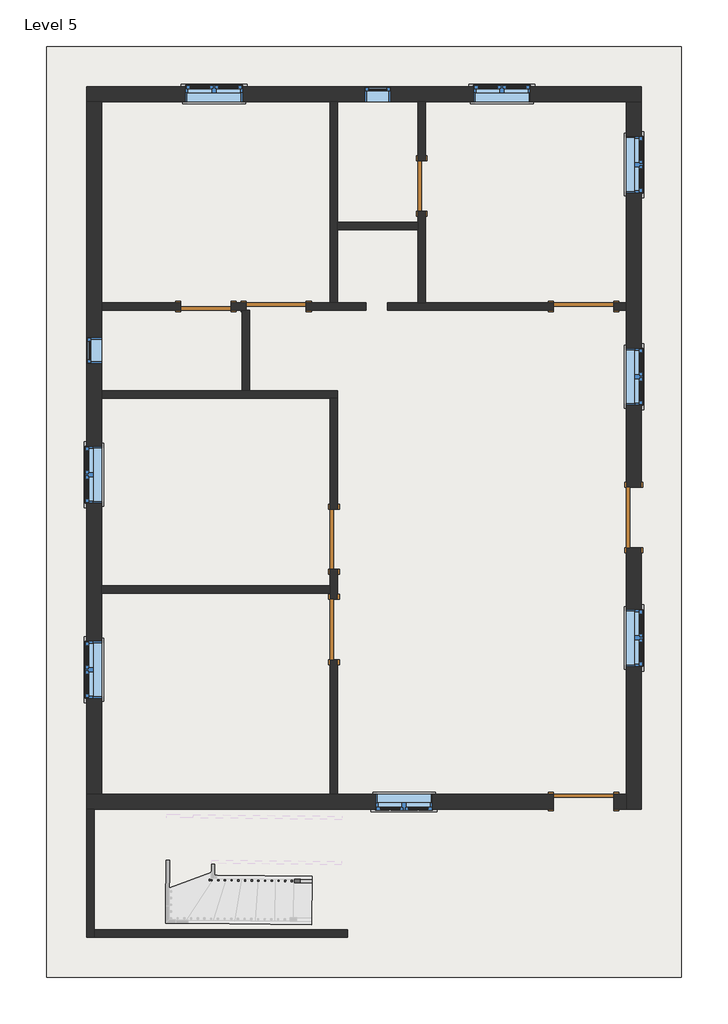
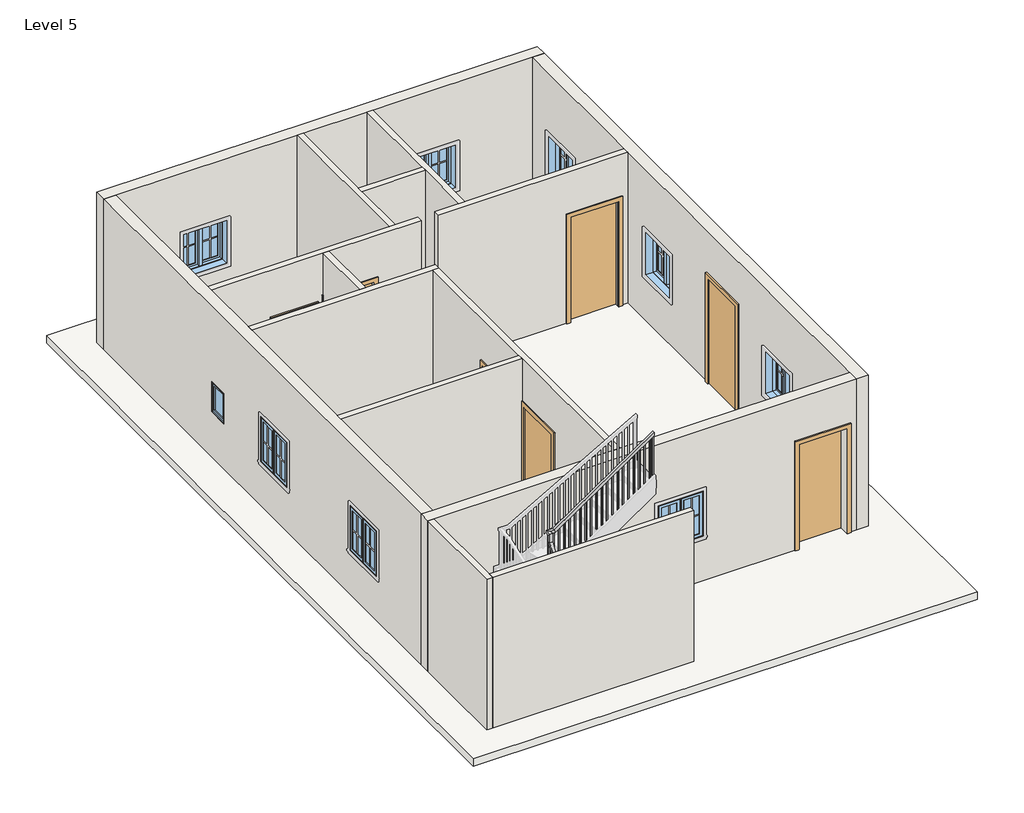
# One storey, part 1 of 2: 15 walls, 10 windows, 8 doors, 1 railing, 1 roof.
"""IFC4 building model written with IfcOpenShell, lengths in millimetres."""

from ifc_helpers import new_model, si_unit, frame, origin, place, context, project, spatial, polyline, outline, extrude, faceted_brep, transform, mapped, element, save
from components import door_f2b275c1, door_e5f9f3c4, door_305aa2a5, door_a90ba1ad, door_0ca8825f, window_aa618e30, window_339605e1

model = new_model("IFC4")

# Units and contexts
model_context = context("Model", 3, world=origin())
ifc_project = project(units=[si_unit("LENGTHUNIT", "METRE", prefix="MILLI")], contexts=[model_context])

# Site, building, storey
site = spatial("IfcSite", under=ifc_project)
building = spatial("IfcBuilding", under=site)
storey = spatial("IfcBuildingStorey", under=building, Name="Level 5", Elevation=9601.2)

# Doors
placement = place(None, origin())
door_shape = door_f2b275c1(model_context)
element("IfcDoor", 1, ObjectType="Single-Flush : 30\" x 80\"", at=placement, inside=storey, context=model_context, shape_type="MappedRepresentation", body=[
    mapped(door_shape, transform((-295.4747832, 5557.2532079, 9601.2), x_axis=(0.0, -1.0, 0.0), y_axis=(1.0, 0.0, 0.0), z_axis=(0.0, 0.0, 1.0))),
])
element("IfcDoor", 2, ObjectType="Single-Flush : 30\" x 80\"", at=placement, inside=storey, context=model_context, shape_type="MappedRepresentation", body=[
    mapped(door_shape, transform((-3572.0747832, 3728.4532079, 9601.2), x_axis=(1.0, 0.0, 0.0), y_axis=(0.0, 1.0, 0.0), z_axis=(0.0, 0.0, 1.0))),
])
door_2_shape = door_e5f9f3c4(model_context)
element("IfcDoor", 3, ObjectType="Single-Flush : 36\" x 84\"", at=placement, inside=storey, context=model_context, shape_type="MappedRepresentation", body=[
    mapped(door_2_shape, transform((-2505.2747832, 3728.4532079, 9601.2), x_axis=(1.0, 0.0, 0.0), y_axis=(0.0, 1.0, 0.0), z_axis=(0.0, 0.0, 1.0))),
])
element("IfcDoor", 4, ObjectType="Single-Flush : 36\" x 84\"", at=placement, inside=storey, context=model_context, shape_type="MappedRepresentation", body=[
    mapped(door_2_shape, transform((2161.9752168, 3728.4532079, 9601.2), x_axis=(1.0, 0.0, 0.0), y_axis=(0.0, 1.0, 0.0), z_axis=(0.0, 0.0, 1.0))),
])
element("IfcDoor", 5, ObjectType="Single-Flush : 36\" x 84\"", at=placement, inside=storey, context=model_context, shape_type="MappedRepresentation", body=[
    mapped(door_2_shape, transform((-1628.9747832, -1173.7467921, 9601.2), x_axis=(0.0, 1.0, 0.0), y_axis=(-1.0, 0.0, 0.0), z_axis=(0.0, 0.0, 1.0))),
])
door_3_shape = door_305aa2a5(model_context)
element("IfcDoor", 6, ObjectType="Single-Flush : 36\" x 84\"", at=placement, inside=storey, context=model_context, shape_type="MappedRepresentation", body=[
    mapped(door_3_shape, transform((-1628.9747832, 197.8532079, 9601.2), x_axis=(0.0, -1.0, 0.0), y_axis=(1.0, 0.0, 0.0), z_axis=(0.0, 0.0, 1.0))),
])
door_4_shape = door_a90ba1ad(model_context)
element("IfcDoor", 7, ObjectType="Single-Flush : 36\" x 84\"", at=placement, inside=storey, context=model_context, shape_type="MappedRepresentation", body=[
    mapped(door_4_shape, transform((2923.9752168, 528.0532079, 9601.2), x_axis=(0.0, -1.0, 0.0), y_axis=(1.0, 0.0, 0.0), z_axis=(0.0, 0.0, 1.0))),
])
door_5_shape = door_0ca8825f(model_context)
element("IfcDoor", 8, ObjectType="Single-Flush : 36\" x 84\"", at=placement, inside=storey, context=model_context, shape_type="MappedRepresentation", body=[
    mapped(door_5_shape, transform((2161.9752168, -3783.5967921, 9601.2), x_axis=(1.0, 0.0, 0.0), y_axis=(0.0, 1.0, 0.0), z_axis=(0.0, 0.0, 1.0))),
])

# Railing
element("IfcRailing", 9, ObjectType="Handrail - Rectangular", at=placement, inside=storey, context=model_context, shape_type="SolidModel", body=[
    faceted_brep([(-1962.1803506, -5016.2038017, 10684.9333333), (-1962.1803506, -5016.2038017, 10623.4793596), (-1961.6349602, -4965.4067295, 10623.4793596), (-1961.6349602, -4965.4067295, 10684.9333333), (-3413.6283866, -5000.6201116, 11673.0756169), (-3464.4254588, -5000.0747212, 11646.2041661), (-3463.8800684, -4949.2776489, 11646.2041661), (-3413.0829962, -4949.8230393, 11673.0756169), (-3413.6283866, -5000.6201116, 11890.161538), (-3464.4254588, -5000.0747212, 11839.361538), (-3463.8800684, -4949.2776489, 11839.361538), (-3413.0829962, -4949.8230393, 11890.161538), (-3540.6210672, -4999.2566356, 11890.161538), (-3540.6210672, -4999.2566356, 11839.361538), (-3489.2786045, -4949.0049537, 11839.361538), (-3489.2786045, -4949.0049537, 11890.161538), (-3539.2575912, -4872.2639549, 11890.161538), (-3538.9677931, -4845.272478, 11839.361538), (-3488.1707209, -4845.8178684, 11839.361538), (-3488.4605189, -4872.8093453, 11890.161538), (-3537.8941152, -4745.2712743, 12078.2249579), (-3537.3487248, -4694.4742021, 12062.6786564), (-3486.5516525, -4695.0195925, 12062.6786564), (-3487.0970429, -4745.8166647, 12078.2249579), (-3537.8941152, -4745.2712743, 12246.276961), (-3537.3487248, -4694.4742021, 12195.476961), (-3486.5516525, -4695.0195925, 12195.476961), (-3487.0970429, -4745.8166647, 12246.276961), (-3536.5306392, -4618.2785937, 12246.276961), (-3536.5306392, -4618.2785937, 12195.476961), (-3486.2789573, -4669.6210563, 12195.476961), (-3486.2789573, -4669.6210563, 12246.276961), (-3409.5379585, -4619.6420697, 12246.276961), (-3393.6525863, -4619.8126254, 12195.476961), (-3394.1979767, -4670.6096976, 12195.476961), (-3410.0833489, -4670.439142, 12246.276961), (-1509.4062983, -4640.0431191, 13563.6), (-1509.9516887, -4690.8401913, 13563.6), (-1509.9516887, -4690.8401913, 13501.7869912), (-1509.4062983, -4640.0431191, 13501.7869912)], [[[0, 1, 2, 3]], [[1, 0, 4, 5]], [[2, 1, 5, 6]], [[3, 2, 6, 7]], [[0, 3, 7, 4]], [[5, 4, 8, 9]], [[6, 5, 9, 10]], [[7, 6, 10, 11]], [[4, 7, 11, 8]], [[9, 8, 12, 13]], [[10, 9, 13, 14]], [[11, 10, 14, 15]], [[8, 11, 15, 12]], [[13, 12, 16, 17]], [[14, 13, 17, 18]], [[15, 14, 18, 19]], [[12, 15, 19, 16]], [[17, 16, 20, 21]], [[18, 17, 21, 22]], [[19, 18, 22, 23]], [[16, 19, 23, 20]], [[21, 20, 24, 25]], [[22, 21, 25, 26]], [[23, 22, 26, 27]], [[20, 23, 27, 24]], [[25, 24, 28, 29]], [[26, 25, 29, 30]], [[27, 26, 30, 31]], [[24, 27, 31, 28]], [[29, 28, 32, 33]], [[30, 29, 33, 34]], [[31, 30, 34, 35]], [[28, 31, 35, 32]], [[36, 37, 38, 39]], [[33, 32, 36, 39]], [[34, 33, 39, 38]], [[35, 34, 38, 37]], [[32, 35, 37, 36]]]),
    extrude(outline(polyline([(221.9968897, -19.05), (235.2031102, 0.0), (1200.994449, 0.0), (1200.994449, -19.05), (221.9968897, -19.05)])), frame((-1590.7427644, -4674.0968508, 13680.8611157), z_axis=(0.01073603161956521, 0.9999423671517594, 0.0), x_axis=(0.0, 0.0, -1.0)), (0.0, 0.0, 1.0), 19.05),
    extrude(outline(polyline([(221.9968898, -19.05), (235.2031102, 0.0), (1130.5612733, 0.0), (1130.5612733, -19.05), (221.9968898, -19.05)])), frame((-1692.3369089, -4673.00607, 13610.42794), z_axis=(0.01073603161956521, 0.9999423671517594, 0.0), x_axis=(0.0, 0.0, -1.0)), (0.0, 0.0, 1.0), 19.05),
    extrude(outline(polyline([(221.9968897, -19.05), (235.2031102, 0.0), (1060.1280975, 0.0), (1060.1280975, -19.05), (221.9968897, -19.05)])), frame((-1793.9310534, -4671.9152892, 13539.9947642), z_axis=(0.01073603161956521, 0.9999423671517594, 0.0), x_axis=(0.0, 0.0, -1.0)), (0.0, 0.0, 1.0), 19.05),
    extrude(outline(polyline([(221.9968898, -19.05), (235.2031103, 0.0), (1159.0282552, 0.0), (1159.0282552, -19.05), (221.9968898, -19.05)])), frame((-1895.5251979, -4670.8245084, 13469.5615885), z_axis=(0.01073603161956521, 0.9999423671517594, 0.0), x_axis=(0.0, 0.0, -1.0)), (0.0, 0.0, 1.0), 19.05),
    extrude(outline(polyline([(221.9968898, -19.05), (235.2031102, 0.0), (1088.5950794, 0.0), (1088.5950794, -19.05), (221.9968898, -19.05)])), frame((-1997.1193424, -4669.7337275, 13399.1284127), z_axis=(0.01073603161956521, 0.9999423671517594, 0.0), x_axis=(0.0, 0.0, -1.0)), (0.0, 0.0, 1.0), 19.05),
    extrude(outline(polyline([(221.9968898, -19.05), (235.2031103, 0.0), (1187.495237, 0.0), (1187.495237, -19.05), (221.9968898, -19.05)])), frame((-2098.7134869, -4668.6429467, 13328.695237), z_axis=(0.01073603161956521, 0.9999423671517594, 0.0), x_axis=(0.0, 0.0, -1.0)), (0.0, 0.0, 1.0), 19.05),
    extrude(outline(polyline([(221.9968898, -19.05), (235.2031102, 0.0), (1117.0620612, 0.0), (1117.0620612, -19.05), (221.9968898, -19.05)])), frame((-2200.3076314, -4667.5521659, 13258.2620612), z_axis=(0.01073603161956521, 0.9999423671517594, 0.0), x_axis=(0.0, 0.0, -1.0)), (0.0, 0.0, 1.0), 19.05),
    extrude(outline(polyline([(221.9968897, -19.0499999), (235.2031102, 0.0), (1046.6288854, 0.0), (1046.6288854, -19.0499999), (221.9968897, -19.0499999)])), frame((-2301.9017759, -4666.4613851, 13187.8288854), z_axis=(0.01073603161956521, 0.9999423671517594, 0.0), x_axis=(0.0, 0.0, -1.0)), (0.0, 0.0, 1.0), 19.05),
    extrude(outline(polyline([(221.9968898, -19.0499999), (235.2031102, 0.0), (1145.529043, 0.0), (1145.529043, -19.0499999), (221.9968898, -19.0499999)])), frame((-2403.4959204, -4665.3706043, 13117.3957097), z_axis=(0.01073603161956521, 0.9999423671517594, 0.0), x_axis=(0.0, 0.0, -1.0)), (0.0, 0.0, 1.0), 19.05),
    extrude(outline(polyline([(221.9968897, -19.05), (235.2031102, 0.0), (1075.0958672, 0.0), (1075.0958672, -19.05), (221.9968897, -19.05)])), frame((-2505.090065, -4664.2798235, 13046.9625339), z_axis=(0.01073603161956521, 0.9999423671517594, 0.0), x_axis=(0.0, 0.0, -1.0)), (0.0, 0.0, 1.0), 19.05),
    extrude(outline(polyline([(221.9968898, -19.05), (235.2031103, 0.0), (1004.6626915, 0.0), (1004.6626915, -19.05), (221.9968898, -19.05)])), frame((-2606.6842095, -4663.1890427, 12976.5293582), z_axis=(0.01073603161956521, 0.9999423671517594, 0.0), x_axis=(0.0, 0.0, -1.0)), (0.0, 0.0, 1.0), 19.05),
    extrude(outline(polyline([(221.9968898, -19.05), (235.2031102, 0.0), (1103.5628491, 0.0), (1103.5628491, -19.05), (221.9968898, -19.05)])), frame((-2708.278354, -4662.0982619, 12906.0961824), z_axis=(0.01073603161956521, 0.9999423671517594, 0.0), x_axis=(0.0, 0.0, -1.0)), (0.0, 0.0, 1.0), 19.05),
    extrude(outline(polyline([(221.9968898, -19.05), (235.2031103, 0.0), (1033.1296734, 0.0), (1033.1296734, -19.05), (221.9968898, -19.05)])), frame((-2809.8724985, -4661.007481, 12835.6630067), z_axis=(0.01073603161956521, 0.9999423671517594, 0.0), x_axis=(0.0, 0.0, -1.0)), (0.0, 0.0, 1.0), 19.05),
    extrude(outline(polyline([(221.9968898, -19.05), (235.2031102, 0.0), (1132.0298309, 0.0), (1132.0298309, -19.05), (221.9968898, -19.05)])), frame((-2911.466643, -4659.9167002, 12765.2298309), z_axis=(0.01073603161956521, 0.9999423671517594, 0.0), x_axis=(0.0, 0.0, -1.0)), (0.0, 0.0, 1.0), 19.05),
    extrude(outline(polyline([(221.9968897, -19.05), (235.2031102, 0.0), (1061.5966551, 0.0), (1061.5966551, -19.05), (221.9968897, -19.05)])), frame((-3013.0607875, -4658.8259194, 12694.7966551), z_axis=(0.01073603161956521, 0.9999423671517594, 0.0), x_axis=(0.0, 0.0, -1.0)), (0.0, 0.0, 1.0), 19.05),
    extrude(outline(polyline([(221.9968898, -19.05), (235.2031102, 0.0), (991.1634794, 0.0), (991.1634794, -19.05), (221.9968898, -19.05)])), frame((-3114.654932, -4657.7351386, 12624.3634794), z_axis=(0.01073603161956521, 0.9999423671517594, 0.0), x_axis=(0.0, 0.0, -1.0)), (0.0, 0.0, 1.0), 19.05),
    extrude(outline(polyline([(221.9968897, -19.05), (235.2031102, 0.0), (1090.0636369, 0.0), (1090.0636369, -19.05), (221.9968897, -19.05)])), frame((-3216.2490765, -4656.6443578, 12553.9303036), z_axis=(0.01073603161956521, 0.9999423671517594, 0.0), x_axis=(0.0, 0.0, -1.0)), (0.0, 0.0, 1.0), 19.05),
    extrude(outline(polyline([(221.9968898, -19.05), (235.2031103, 0.0), (1019.6304612, 0.0), (1019.6304612, -19.05), (221.9968898, -19.05)])), frame((-3317.843221, -4655.553577, 12483.4971279), z_axis=(0.01073603161956521, 0.9999423671517594, 0.0), x_axis=(0.0, 0.0, -1.0)), (0.0, 0.0, 1.0), 19.05),
    extrude(outline(polyline([(221.9968898, -19.05), (235.2031102, 0.0), (1118.5306188, 0.0), (1118.5306188, -19.05), (221.9968898, -19.05)])), frame((-3419.4373655, -4654.4627962, 12413.0639521), z_axis=(0.01073603161956521, 0.9999423671517594, 0.0), x_axis=(0.0, 0.0, -1.0)), (0.0, 0.0, 1.0), 19.05),
    extrude(outline(polyline([(-3502.2553031, -4678.9750729), (-3521.3042052, -4678.7705515), (-3521.0996838, -4659.7216494), (-3502.0507817, -4659.9261708), (-3502.2553031, -4678.9750729)])), frame((0.0, 0.0, 11125.2), z_axis=(0.0, 0.0, 1.0), x_axis=(1.0, 0.0, 0.0)), (0.0, 0.0, 1.0), 1070.276961),
    extrude(outline(polyline([(214.4952435, -19.05), (242.7047565, 0.0), (1222.5739377, 0.0), (1222.5739377, -19.05), (214.4952435, -19.05)])), frame((-3503.3460839, -4780.5692174, 12178.4406044), z_axis=(-0.9999423671517594, 0.010736031619565895, 0.0), x_axis=(0.0, 0.0, -1.0)), (0.0, 0.0, 1.0), 19.05),
    extrude(outline(polyline([(214.4952435, -19.05), (242.7047565, 0.0), (1072.1232018, 0.0), (1072.1232018, -19.05), (214.4952435, -19.05)])), frame((-3504.4368647, -4882.1633619, 12027.9898685), z_axis=(-0.9999423671517594, 0.010736031619565895, 0.0), x_axis=(0.0, 0.0, -1.0)), (0.0, 0.0, 1.0), 19.05),
    extrude(outline(polyline([(-3476.1931112, -4965.0213631), (-3476.3976326, -4984.0702652), (-3495.4465347, -4983.8657438), (-3495.2420133, -4964.8168417), (-3476.1931112, -4965.0213631)])), frame((0.0, 0.0, 10786.5333333), z_axis=(0.0, 0.0, 1.0), x_axis=(1.0, 0.0, 0.0)), (0.0, 0.0, 1.0), 1052.8282047),
    extrude(outline(polyline([(235.0842231, -19.05), (222.115777, 0.0), (1203.1900014, 0.0), (1203.1900014, -19.05), (235.0842231, -19.05)])), frame((-3393.8523902, -4984.9565246, 11820.3900014), z_axis=(0.01073603161956537, 0.9999423671517593, 0.0), x_axis=(0.0, 0.0, -1.0)), (0.0, 0.0, 1.0), 19.05),
    extrude(outline(polyline([(235.084223, -19.05), (222.1157769, 0.0), (1134.0249555, 0.0), (1134.0249555, -19.05), (235.084223, -19.05)])), frame((-3292.2582457, -4986.0473054, 11751.2249555), z_axis=(0.01073603161956537, 0.9999423671517593, 0.0), x_axis=(0.0, 0.0, -1.0)), (0.0, 0.0, 1.0), 19.05),
    extrude(outline(polyline([(235.0842231, -19.05), (222.115777, 0.0), (1234.193243, 0.0), (1234.193243, -19.05), (235.0842231, -19.05)])), frame((-3190.6641012, -4987.1380862, 11682.0599097), z_axis=(0.01073603161956537, 0.9999423671517593, 0.0), x_axis=(0.0, 0.0, -1.0)), (0.0, 0.0, 1.0), 19.05),
    extrude(outline(polyline([(235.084223, -19.05), (222.1157769, 0.0), (1165.0281971, 0.0), (1165.0281971, -19.05), (235.084223, -19.05)])), frame((-3089.0699567, -4988.228867, 11612.8948638), z_axis=(0.01073603161956537, 0.9999423671517593, 0.0), x_axis=(0.0, 0.0, -1.0)), (0.0, 0.0, 1.0), 19.05),
    extrude(outline(polyline([(235.084223, -19.05), (222.1157769, 0.0), (1265.1964847, 0.0), (1265.1964847, -19.05), (235.084223, -19.05)])), frame((-2987.4758122, -4989.3196478, 11543.729818), z_axis=(0.01073603161956537, 0.9999423671517593, 0.0), x_axis=(0.0, 0.0, -1.0)), (0.0, 0.0, 1.0), 19.05),
    extrude(outline(polyline([(235.0842231, -19.05), (222.115777, 0.0), (1196.0314389, 0.0), (1196.0314389, -19.05), (235.0842231, -19.05)])), frame((-2885.8816677, -4990.4104286, 11474.5647722), z_axis=(0.01073603161956537, 0.9999423671517593, 0.0), x_axis=(0.0, 0.0, -1.0)), (0.0, 0.0, 1.0), 19.05),
    extrude(outline(polyline([(235.084223, -19.05), (222.1157769, 0.0), (1296.1997263, 0.0), (1296.1997263, -19.05), (235.084223, -19.05)])), frame((-2784.2875232, -4991.5012094, 11405.3997263), z_axis=(0.01073603161956537, 0.9999423671517593, 0.0), x_axis=(0.0, 0.0, -1.0)), (0.0, 0.0, 1.0), 19.05),
    extrude(outline(polyline([(235.0842231, -19.05), (222.115777, 0.0), (1227.0346805, 0.0), (1227.0346805, -19.05), (235.0842231, -19.05)])), frame((-2682.6933787, -4992.5919903, 11336.2346805), z_axis=(0.01073603161956537, 0.9999423671517593, 0.0), x_axis=(0.0, 0.0, -1.0)), (0.0, 0.0, 1.0), 19.05),
    extrude(outline(polyline([(235.084223, -19.05), (222.1157769, 0.0), (1157.8696346, 0.0), (1157.8696346, -19.05), (235.084223, -19.05)])), frame((-2581.0992342, -4993.6827711, 11267.0696346), z_axis=(0.01073603161956537, 0.9999423671517593, 0.0), x_axis=(0.0, 0.0, -1.0)), (0.0, 0.0, 1.0), 19.05),
    extrude(outline(polyline([(235.0842231, -19.05), (222.115777, 0.0), (1258.0379221, 0.0), (1258.0379221, -19.05), (235.0842231, -19.05)])), frame((-2479.5050897, -4994.7735519, 11197.9045888), z_axis=(0.01073603161956537, 0.9999423671517593, 0.0), x_axis=(0.0, 0.0, -1.0)), (0.0, 0.0, 1.0), 19.05),
    extrude(outline(polyline([(235.084223, -19.05), (222.1157769, 0.0), (1188.8728762, 0.0), (1188.8728762, -19.05), (235.084223, -19.05)])), frame((-2377.9109452, -4995.8643327, 11128.7395429), z_axis=(0.01073603161956537, 0.9999423671517593, 0.0), x_axis=(0.0, 0.0, -1.0)), (0.0, 0.0, 1.0), 19.05),
    extrude(outline(polyline([(235.084223, -19.05), (222.115777, 0.0), (1119.7078304, 0.0), (1119.7078304, -19.05), (235.084223, -19.05)])), frame((-2276.3168007, -4996.9551135, 11059.5744971), z_axis=(0.01073603161956537, 0.9999423671517593, 0.0), x_axis=(0.0, 0.0, -1.0)), (0.0, 0.0, 1.0), 19.05),
    extrude(outline(polyline([(235.0842231, -19.05), (222.115777, 0.0), (1219.876118, 0.0), (1219.876118, -19.05), (235.0842231, -19.05)])), frame((-2174.7226562, -4998.0458943, 10990.4094513), z_axis=(0.01073603161956537, 0.9999423671517593, 0.0), x_axis=(0.0, 0.0, -1.0)), (0.0, 0.0, 1.0), 19.05),
    extrude(outline(polyline([(235.084223, -19.05), (222.1157769, 0.0), (1150.7110721, 0.0), (1150.7110721, -19.05), (235.084223, -19.05)])), frame((-2073.1285117, -4999.1366751, 10921.2444054), z_axis=(0.01073603161956537, 0.9999423671517593, 0.0), x_axis=(0.0, 0.0, -1.0)), (0.0, 0.0, 1.0), 19.05),
    extrude(outline(polyline([(-3501.9826079, -4653.5765368), (-3521.03151, -4653.3720154), (-3520.8269886, -4634.3231133), (-3501.7780865, -4634.5276347), (-3501.9826079, -4653.5765368)])), frame((0.0, 0.0, 11125.2), z_axis=(0.0, 0.0, 1.0), x_axis=(1.0, 0.0, 0.0)), (0.0, 0.0, 1.0), 1070.276961),
    extrude(outline(polyline([(-3505.3231241, -4964.7086043), (-3505.5276455, -4983.7575064), (-3524.5765476, -4983.552985), (-3524.3720262, -4964.5040829), (-3505.3231241, -4964.7086043)])), frame((0.0, 0.0, 10786.5333333), z_axis=(0.0, 0.0, 1.0), x_axis=(1.0, 0.0, 0.0)), (0.0, 0.0, 1.0), 1052.8282047),
    extrude(outline(polyline([(221.9968897, -19.05), (235.2031102, 0.0), (1243.9172142, 0.0), (1243.9172142, -19.05), (221.9968897, -19.05)])), frame((-1528.8301563, -4674.7615848, 13723.7838809), z_axis=(0.01073603161956521, 0.9999423671517594, 0.0), x_axis=(0.0, 0.0, -1.0)), (0.0, 0.0, 1.0), 19.05),
    extrude(outline(polyline([(235.084223, -19.05), (222.1157769, 0.0), (1088.0302493, 0.0), (1088.0302493, -19.05), (235.084223, -19.05)])), frame((-1981.0588182, -5000.1251952, 10858.5635826), z_axis=(0.01073603161956537, 0.9999423671517593, 0.0), x_axis=(0.0, 0.0, -1.0)), (0.0, 0.0, 1.0), 19.05),
])

# Roof
element("IfcRoof", 10, ObjectType="Generic - 12\"", at=placement, inside=storey, context=model_context, shape_type="SweptSolid", body=[
    extrude(outline(polyline([(-5991.4247832, 7671.8032079), (3647.8752168, 7671.8032079), (3647.8752168, -6450.5967921), (-5991.4247832, -6450.5967921), (-5991.4247832, 7671.8032079)])), frame((0.0, 0.0, 9448.8), z_axis=(0.0, 0.0, 1.0), x_axis=(1.0, 0.0, 0.0)), (0.0, 0.0, 1.0), 152.4),
])

# Walls
element("IfcWall", 11, ObjectType="WALL4.5\"", at=placement, inside=storey, context=model_context, shape_type="Brep", body=[
    faceted_brep([(-2048.0747832, 3671.3032079, 11734.8), (-2048.0747832, 3671.3032079, 9601.2), (-1141.0287494, 3671.3032079, 9601.2), (-1141.0287494, 3671.3032079, 12649.2), (-2905.3247832, 3671.3032079, 12649.2), (-3019.6247832, 3671.3032079, 12649.2), (-5153.2247832, 3671.3032079, 12649.2), (-5153.2247832, 3671.3032079, 9601.2), (-3953.0747832, 3671.3032079, 9601.2), (-3953.0747832, 3671.3032079, 11633.2), (-3191.0747832, 3671.3032079, 11633.2), (-3191.0747832, 3671.3032079, 9601.2), (-3019.6247832, 3671.3032079, 9601.2), (-2962.4747832, 3671.3032079, 9601.2), (-2962.4747832, 3671.3032079, 11734.8), (-1141.0287494, 3785.6032079, 9601.2), (-1571.8247832, 3785.6032079, 9601.2), (-1686.1247832, 3785.6032079, 9601.2), (-2048.0747832, 3785.6032079, 9601.2), (-2048.0747832, 3785.6032079, 11734.8), (-2962.4747832, 3785.6032079, 11734.8), (-2962.4747832, 3785.6032079, 9601.2), (-3191.0747832, 3785.6032079, 9601.2), (-3191.0747832, 3785.6032079, 11633.2), (-3953.0747832, 3785.6032079, 11633.2), (-3953.0747832, 3785.6032079, 9601.2), (-5153.2247832, 3785.6032079, 9601.2), (-5153.2247832, 3785.6032079, 12649.2), (-1686.1247832, 3785.6032079, 12649.2), (-1571.8247832, 3785.6032079, 12649.2), (-1141.0287494, 3785.6032079, 12649.2)], [[[0, 1, 2, 3, 4, 5, 6, 7, 8, 9, 10, 11, 12, 13, 14]], [[15, 16, 17, 18, 19, 20, 21, 22, 23, 24, 25, 26, 27, 28, 29, 30]], [[8, 7, 26, 25]], [[2, 1, 18, 17, 16, 15]], [[13, 12, 11, 22, 21]], [[3, 2, 15, 30]], [[7, 6, 27, 26]], [[23, 22, 11, 10]], [[24, 23, 10, 9]], [[25, 24, 9, 8]], [[19, 18, 1, 0]], [[20, 19, 0, 14]], [[21, 20, 14, 13]], [[6, 5, 4, 3, 30, 29, 28, 27]]]),
])
element("IfcWall", 12, ObjectType="WALL4.5\"", at=placement, inside=storey, context=model_context, shape_type="Brep", body=[
    faceted_brep([(2619.1752168, 3671.3032079, 11734.8), (2619.1752168, 3671.3032079, 9601.2), (2809.6752168, 3671.3032079, 9601.2), (2809.6752168, 3671.3032079, 12649.2), (-812.7163761, 3671.3032079, 12649.2), (-812.7163761, 3671.3032079, 9601.2), (1704.7752168, 3671.3032079, 9601.2), (1704.7752168, 3671.3032079, 11734.8), (2809.6752168, 3785.6032079, 9601.2), (2619.1752168, 3785.6032079, 9601.2), (2619.1752168, 3785.6032079, 11734.8), (1704.7752168, 3785.6032079, 11734.8), (1704.7752168, 3785.6032079, 9601.2), (-238.3247832, 3785.6032079, 9601.2), (-352.6247832, 3785.6032079, 9601.2), (-812.7163761, 3785.6032079, 9601.2), (-812.7163761, 3785.6032079, 12649.2), (-352.6247832, 3785.6032079, 12649.2), (-238.3247832, 3785.6032079, 12649.2), (2809.6752168, 3785.6032079, 12649.2)], [[[0, 1, 2, 3, 4, 5, 6, 7]], [[8, 9, 10, 11, 12, 13, 14, 15, 16, 17, 18, 19]], [[6, 5, 15, 14, 13, 12]], [[2, 1, 9, 8]], [[5, 4, 16, 15]], [[3, 2, 8, 19]], [[10, 9, 1, 0]], [[11, 10, 0, 7]], [[12, 11, 7, 6]], [[4, 3, 19, 18, 17, 16]]]),
])
element("IfcWall", 13, ObjectType="WALL4.5\"", at=placement, inside=storey, context=model_context, shape_type="Brep", body=[
    faceted_brep([(-1686.1247832, 6833.6032079, 9601.2), (-1686.1247832, 3785.6032079, 9601.2), (-1686.1247832, 3785.6032079, 12649.2), (-1686.1247832, 6833.6032079, 12649.2), (-1571.8247832, 6833.6032079, 9601.2), (-1571.8247832, 6833.6032079, 12649.2), (-1571.8247832, 5004.8032079, 12649.2), (-1571.8247832, 4890.5032079, 12649.2), (-1571.8247832, 3785.6032079, 12649.2), (-1571.8247832, 3785.6032079, 9601.2), (-1571.8247832, 4890.5032079, 9601.2), (-1571.8247832, 5004.8032079, 9601.2)], [[[0, 1, 2, 3]], [[4, 5, 6, 7, 8, 9, 10, 11]], [[1, 0, 4, 11, 10, 9]], [[0, 3, 5, 4]], [[2, 1, 9, 8]], [[3, 2, 8, 7, 6, 5]]]),
])
element("IfcWall", 14, ObjectType="WALL4.5\"", at=placement, inside=storey, context=model_context, shape_type="SweptSolid", body=[
    extrude(outline(polyline([(-352.6247832, 4890.5032079), (-1571.8247832, 4890.5032079), (-1571.8247832, 5004.8032079), (-352.6247832, 5004.8032079), (-352.6247832, 4890.5032079)])), frame((0.0, 0.0, 9601.2), z_axis=(0.0, 0.0, 1.0), x_axis=(1.0, 0.0, 0.0)), (0.0, 0.0, 1.0), 3048.0),
])
element("IfcWall", 15, ObjectType="WALL4.5\"", at=placement, inside=storey, context=model_context, shape_type="Brep", body=[
    faceted_brep([(-352.6247832, 5176.2532079, 11633.2), (-352.6247832, 5176.2532079, 9601.2), (-352.6247832, 5004.8032079, 9601.2), (-352.6247832, 4890.5032079, 9601.2), (-352.6247832, 3785.6032079, 9601.2), (-352.6247832, 3785.6032079, 12649.2), (-352.6247832, 4890.5032079, 12649.2), (-352.6247832, 5004.8032079, 12649.2), (-352.6247832, 6833.6032079, 12649.2), (-352.6247832, 6833.6032079, 9601.2), (-352.6247832, 5938.2532079, 9601.2), (-352.6247832, 5938.2532079, 11633.2), (-238.3247832, 3785.6032079, 9601.2), (-238.3247832, 5176.2532079, 9601.2), (-238.3247832, 5176.2532079, 11633.2), (-238.3247832, 5938.2532079, 11633.2), (-238.3247832, 5938.2532079, 9601.2), (-238.3247832, 6833.6032079, 9601.2), (-238.3247832, 6833.6032079, 12649.2), (-238.3247832, 3785.6032079, 12649.2)], [[[0, 1, 2, 3, 4, 5, 6, 7, 8, 9, 10, 11]], [[12, 13, 14, 15, 16, 17, 18, 19]], [[10, 9, 17, 16]], [[4, 3, 2, 1, 13, 12]], [[9, 8, 18, 17]], [[5, 4, 12, 19]], [[14, 13, 1, 0]], [[15, 14, 0, 11]], [[16, 15, 11, 10]], [[8, 7, 6, 5, 19, 18]]]),
])
element("IfcWall", 16, ObjectType="WALL4.5\"", at=placement, inside=storey, context=model_context, shape_type="Brep", body=[
    faceted_brep([(-3019.6247832, 3671.3032079, 9601.2), (-3019.6247832, 2452.1032079, 9601.2), (-3019.6247832, 2452.1032079, 12649.2), (-3019.6247832, 3671.3032079, 12649.2), (-2905.3247832, 3671.3032079, 9601.2), (-2905.3247832, 3671.3032079, 12649.2), (-2905.3247832, 2452.1032079, 12649.2), (-2905.3247832, 2452.1032079, 9601.2), (-2962.4747832, 3671.3032079, 9601.2)], [[[0, 1, 2, 3]], [[4, 5, 6, 7]], [[1, 0, 8, 4, 7]], [[0, 3, 5, 4, 8]], [[2, 1, 7, 6]], [[3, 2, 6, 5]]]),
])
element("IfcWall", 17, ObjectType="WALL4.5\"", at=placement, inside=storey, context=model_context, shape_type="Brep", body=[
    faceted_brep([(-5153.2247832, 2337.8032079, 9601.2), (-1686.1247832, 2337.8032079, 9601.2), (-1571.8247832, 2337.8032079, 9601.2), (-1571.8247832, 2337.8032079, 12649.2), (-1686.1247832, 2337.8032079, 12649.2), (-5153.2247832, 2337.8032079, 12649.2), (-5153.2247832, 2452.1032079, 9601.2), (-5153.2247832, 2452.1032079, 12649.2), (-3019.6247832, 2452.1032079, 12649.2), (-2905.3247832, 2452.1032079, 12649.2), (-1571.8247832, 2452.1032079, 12649.2), (-1571.8247832, 2452.1032079, 9601.2), (-2905.3247832, 2452.1032079, 9601.2), (-3019.6247832, 2452.1032079, 9601.2)], [[[0, 1, 2, 3, 4, 5]], [[6, 7, 8, 9, 10, 11, 12, 13]], [[2, 1, 0, 6, 13, 12, 11]], [[0, 5, 7, 6]], [[3, 2, 11, 10]], [[5, 4, 3, 10, 9, 8, 7]]]),
])
element("IfcWall", 18, ObjectType="WALL4.5\"", at=placement, inside=storey, context=model_context, shape_type="Brep", body=[
    faceted_brep([(-1686.1247832, -259.3467921, 9601.2), (-1686.1247832, -506.9967921, 9601.2), (-1686.1247832, -621.2967921, 9601.2), (-1686.1247832, -716.5467921, 9601.2), (-1686.1247832, -716.5467921, 11734.8), (-1686.1247832, -1630.9467921, 11734.8), (-1686.1247832, -1630.9467921, 9601.2), (-1686.1247832, -3669.2967921, 9601.2), (-1686.1247832, -3669.2967921, 12649.2), (-1686.1247832, -621.2967921, 12649.2), (-1686.1247832, -506.9967921, 12649.2), (-1686.1247832, 2337.8032079, 12649.2), (-1686.1247832, 2337.8032079, 9601.2), (-1686.1247832, 655.0532079, 9601.2), (-1686.1247832, 655.0532079, 11734.8), (-1686.1247832, -259.3467921, 11734.8), (-1571.8247832, -716.5467921, 11734.8), (-1571.8247832, -716.5467921, 9601.2), (-1571.8247832, -259.3467921, 9601.2), (-1571.8247832, -259.3467921, 11734.8), (-1571.8247832, 655.0532079, 11734.8), (-1571.8247832, 655.0532079, 9601.2), (-1571.8247832, 2337.8032079, 9601.2), (-1571.8247832, 2337.8032079, 12649.2), (-1571.8247832, -3669.2967921, 12649.2), (-1571.8247832, -3669.2967921, 9601.2), (-1571.8247832, -1630.9467921, 9601.2), (-1571.8247832, -1630.9467921, 11734.8)], [[[0, 1, 2, 3, 4, 5, 6, 7, 8, 9, 10, 11, 12, 13, 14, 15]], [[16, 17, 18, 19, 20, 21, 22, 23, 24, 25, 26, 27]], [[13, 12, 22, 21]], [[26, 25, 7, 6]], [[18, 17, 3, 2, 1, 0]], [[12, 11, 23, 22]], [[8, 7, 25, 24]], [[19, 18, 0, 15]], [[20, 19, 15, 14]], [[21, 20, 14, 13]], [[4, 3, 17, 16]], [[5, 4, 16, 27]], [[6, 5, 27, 26]], [[11, 10, 9, 8, 24, 23]]]),
])
element("IfcWall", 19, ObjectType="WALL4.5\"", at=placement, inside=storey, context=model_context, shape_type="SweptSolid", body=[
    extrude(outline(polyline([(-1686.1247832, -621.2967921), (-5153.2247832, -621.2967921), (-5153.2247832, -506.9967921), (-1686.1247832, -506.9967921), (-1686.1247832, -621.2967921)])), frame((0.0, 0.0, 9601.2), z_axis=(0.0, 0.0, 1.0), x_axis=(1.0, 0.0, 0.0)), (0.0, 0.0, 1.0), 3048.0),
])
element("IfcWall", 20, ObjectType="WALL4.5\"", at=placement, inside=storey, context=model_context, shape_type="Brep", body=[
    faceted_brep([(-5381.8247832, -3897.8967921, 9601.2), (-5381.8247832, -5840.9967921, 9601.2), (-5381.8247832, -5840.9967921, 12649.2), (-5381.8247832, -3897.8967921, 12649.2), (-5267.5247832, -3897.8967921, 9601.2), (-5267.5247832, -3897.8967921, 12649.2), (-5267.5247832, -5726.6967921, 12649.2), (-5267.5247832, -5840.9967921, 12649.2), (-5267.5247832, -5840.9967921, 9601.2), (-5267.5247832, -5726.6967921, 9601.2)], [[[0, 1, 2, 3]], [[4, 5, 6, 7, 8, 9]], [[1, 0, 4, 9, 8]], [[0, 3, 5, 4]], [[2, 1, 8, 7]], [[3, 2, 7, 6, 5]]]),
])
element("IfcWall", 21, ObjectType="WALL4.5\"", at=placement, inside=storey, context=model_context, shape_type="SweptSolid", body=[
    extrude(outline(polyline([(-1419.4247832, -5840.9967921), (-5267.5247832, -5840.9967921), (-5267.5247832, -5726.6967921), (-1419.4247832, -5726.6967921), (-1419.4247832, -5840.9967921)])), frame((0.0, 0.0, 9601.2), z_axis=(0.0, 0.0, 1.0), x_axis=(1.0, 0.0, 0.0)), (0.0, 0.0, 1.0), 3048.0),
])
element("IfcWall", 22, ObjectType="WALL9\"", at=placement, inside=storey, context=model_context, shape_type="Brep", body=[
    faceted_brep([(-5381.8247832, 6833.6032079, 9601.2), (-5153.2247832, 6833.6032079, 9601.2), (-1686.1247832, 6833.6032079, 9601.2), (-1571.8247832, 6833.6032079, 9601.2), (-352.6247832, 6833.6032079, 9601.2), (-238.3247832, 6833.6032079, 9601.2), (2809.6752168, 6833.6032079, 9601.2), (3038.2752168, 6833.6032079, 9601.2), (3038.2752168, 6833.6032079, 12649.2), (2809.6752168, 6833.6032079, 12649.2), (-238.3247832, 6833.6032079, 12649.2), (-352.6247832, 6833.6032079, 12649.2), (-1571.8247832, 6833.6032079, 12649.2), (-1686.1247832, 6833.6032079, 12649.2), (-5153.2247832, 6833.6032079, 12649.2), (-5381.8247832, 6833.6032079, 12649.2), (-759.0247832, 6833.6032079, 11125.2), (-759.0247832, 6833.6032079, 10515.6), (-1165.4247832, 6833.6032079, 10515.6), (-1165.4247832, 6833.6032079, 11125.2), (-3016.4497832, 6833.6032079, 11430.0), (-3016.4497832, 6833.6032079, 10515.6), (-3880.0497832, 6833.6032079, 10515.6), (-3880.0497832, 6833.6032079, 11430.0), (1355.5252168, 6833.6032079, 11430.0), (1355.5252168, 6833.6032079, 10515.6), (491.9252168, 6833.6032079, 10515.6), (491.9252168, 6833.6032079, 11430.0), (-5381.8247832, 7062.2032079, 9601.2), (-5381.8247832, 7062.2032079, 12649.2), (3038.2752168, 7062.2032079, 12649.2), (3038.2752168, 7062.2032079, 9601.2), (-759.0247832, 7062.2032079, 11125.2), (-1165.4247832, 7062.2032079, 11125.2), (-1165.4247832, 7062.2032079, 10515.6), (-759.0247832, 7062.2032079, 10515.6), (-3016.4497832, 7062.2032079, 11430.0), (-3880.0497832, 7062.2032079, 11430.0), (-3880.0497832, 7062.2032079, 10515.6), (-3016.4497832, 7062.2032079, 10515.6), (1355.5252168, 7062.2032079, 11430.0), (491.9252168, 7062.2032079, 11430.0), (491.9252168, 7062.2032079, 10515.6), (1355.5252168, 7062.2032079, 10515.6)], [[[0, 1, 2, 3, 4, 5, 6, 7, 8, 9, 10, 11, 12, 13, 14, 15], [16, 17, 18, 19], [20, 21, 22, 23], [24, 25, 26, 27]], [[28, 29, 30, 31], [32, 33, 34, 35], [36, 37, 38, 39], [40, 41, 42, 43]], [[7, 6, 5, 4, 3, 2, 1, 0, 28, 31]], [[8, 7, 31, 30]], [[0, 15, 29, 28]], [[17, 16, 32, 35]], [[18, 17, 35, 34]], [[19, 18, 34, 33]], [[16, 19, 33, 32]], [[21, 20, 36, 39]], [[22, 21, 39, 38]], [[23, 22, 38, 37]], [[20, 23, 37, 36]], [[25, 24, 40, 43]], [[26, 25, 43, 42]], [[27, 26, 42, 41]], [[24, 27, 41, 40]], [[15, 14, 13, 12, 11, 10, 9, 8, 30, 29]]]),
])
element("IfcWall", 23, ObjectType="WALL9\"", at=placement, inside=storey, context=model_context, shape_type="Brep", body=[
    faceted_brep([(2809.6752168, 70.8532079, 11734.8), (2809.6752168, 70.8532079, 9601.2), (2809.6752168, -3669.2967921, 9601.2), (2809.6752168, -3897.8967921, 9601.2), (2809.6752168, -3897.8967921, 12649.2), (2809.6752168, -3669.2967921, 12649.2), (2809.6752168, 3671.3032079, 12649.2), (2809.6752168, 3785.6032079, 12649.2), (2809.6752168, 6833.6032079, 12649.2), (2809.6752168, 6833.6032079, 9601.2), (2809.6752168, 3785.6032079, 9601.2), (2809.6752168, 3671.3032079, 9601.2), (2809.6752168, 985.2532079, 9601.2), (2809.6752168, 985.2532079, 11734.8), (2809.6752168, 5449.3032079, 11430.0), (2809.6752168, 5449.3032079, 10515.6), (2809.6752168, 6312.9032079, 10515.6), (2809.6752168, 6312.9032079, 11430.0), (2809.6752168, 2229.8532079, 11430.0), (2809.6752168, 2229.8532079, 10515.6), (2809.6752168, 3093.4532079, 10515.6), (2809.6752168, 3093.4532079, 11430.0), (2809.6752168, -1732.5467921, 11430.0), (2809.6752168, -1732.5467921, 10515.6), (2809.6752168, -868.9467921, 10515.6), (2809.6752168, -868.9467921, 11430.0), (3038.2752168, -3897.8967921, 9601.2), (3038.2752168, 70.8532079, 9601.2), (3038.2752168, 70.8532079, 11734.8), (3038.2752168, 985.2532079, 11734.8), (3038.2752168, 985.2532079, 9601.2), (3038.2752168, 6833.6032079, 9601.2), (3038.2752168, 6833.6032079, 12649.2), (3038.2752168, -3897.8967921, 12649.2), (3038.2752168, 5449.3032079, 11430.0), (3038.2752168, 6312.9032079, 11430.0), (3038.2752168, 6312.9032079, 10515.6), (3038.2752168, 5449.3032079, 10515.6), (3038.2752168, 2229.8532079, 11430.0), (3038.2752168, 3093.4532079, 11430.0), (3038.2752168, 3093.4532079, 10515.6), (3038.2752168, 2229.8532079, 10515.6), (3038.2752168, -1732.5467921, 11430.0), (3038.2752168, -868.9467921, 11430.0), (3038.2752168, -868.9467921, 10515.6), (3038.2752168, -1732.5467921, 10515.6)], [[[0, 1, 2, 3, 4, 5, 6, 7, 8, 9, 10, 11, 12, 13], [14, 15, 16, 17], [18, 19, 20, 21], [22, 23, 24, 25]], [[26, 27, 28, 29, 30, 31, 32, 33], [34, 35, 36, 37], [38, 39, 40, 41], [42, 43, 44, 45]], [[3, 2, 1, 27, 26]], [[12, 11, 10, 9, 31, 30]], [[9, 8, 32, 31]], [[4, 3, 26, 33]], [[28, 27, 1, 0]], [[29, 28, 0, 13]], [[30, 29, 13, 12]], [[15, 14, 34, 37]], [[16, 15, 37, 36]], [[17, 16, 36, 35]], [[14, 17, 35, 34]], [[19, 18, 38, 41]], [[20, 19, 41, 40]], [[21, 20, 40, 39]], [[18, 21, 39, 38]], [[23, 22, 42, 45]], [[24, 23, 45, 44]], [[25, 24, 44, 43]], [[22, 25, 43, 42]], [[8, 7, 6, 5, 4, 33, 32]]]),
])
element("IfcWall", 24, ObjectType="WALL9\"", at=placement, inside=storey, context=model_context, shape_type="Brep", body=[
    faceted_brep([(2809.6752168, -3669.2967921, 9601.2), (2619.1752168, -3669.2967921, 9601.2), (2619.1752168, -3669.2967921, 11734.8), (1704.7752168, -3669.2967921, 11734.8), (1704.7752168, -3669.2967921, 9601.2), (-1571.8247832, -3669.2967921, 9601.2), (-1686.1247832, -3669.2967921, 9601.2), (-5153.2247832, -3669.2967921, 9601.2), (-5381.8247832, -3669.2967921, 9601.2), (-5381.8247832, -3669.2967921, 12649.2), (-5153.2247832, -3669.2967921, 12649.2), (-1686.1247832, -3669.2967921, 12649.2), (-1571.8247832, -3669.2967921, 12649.2), (2809.6752168, -3669.2967921, 12649.2), (-993.9747832, -3669.2967921, 11430.0), (-993.9747832, -3669.2967921, 10515.6), (-130.3747832, -3669.2967921, 10515.6), (-130.3747832, -3669.2967921, 11430.0), (2619.1752168, -3897.8967921, 11734.8), (2619.1752168, -3897.8967921, 9601.2), (2809.6752168, -3897.8967921, 9601.2), (2809.6752168, -3897.8967921, 12649.2), (-5267.5247832, -3897.8967921, 12649.2), (-5381.8247832, -3897.8967921, 12649.2), (-5381.8247832, -3897.8967921, 9601.2), (-5267.5247832, -3897.8967921, 9601.2), (1704.7752168, -3897.8967921, 9601.2), (1704.7752168, -3897.8967921, 11734.8), (-993.9747832, -3897.8967921, 11430.0), (-130.3747832, -3897.8967921, 11430.0), (-130.3747832, -3897.8967921, 10515.6), (-993.9747832, -3897.8967921, 10515.6)], [[[0, 1, 2, 3, 4, 5, 6, 7, 8, 9, 10, 11, 12, 13], [14, 15, 16, 17]], [[18, 19, 20, 21, 22, 23, 24, 25, 26, 27], [28, 29, 30, 31]], [[20, 19, 1, 0]], [[26, 25, 24, 8, 7, 6, 5, 4]], [[0, 13, 21, 20]], [[9, 8, 24, 23]], [[2, 1, 19, 18]], [[3, 2, 18, 27]], [[4, 3, 27, 26]], [[15, 14, 28, 31]], [[16, 15, 31, 30]], [[17, 16, 30, 29]], [[14, 17, 29, 28]], [[13, 12, 11, 10, 9, 23, 22, 21]]]),
])
element("IfcWall", 25, ObjectType="WALL9\"", at=placement, inside=storey, context=model_context, shape_type="Brep", body=[
    faceted_brep([(-5153.2247832, -3669.2967921, 9601.2), (-5153.2247832, -621.2967921, 9601.2), (-5153.2247832, -506.9967921, 9601.2), (-5153.2247832, 2337.8032079, 9601.2), (-5153.2247832, 2452.1032079, 9601.2), (-5153.2247832, 3671.3032079, 9601.2), (-5153.2247832, 3785.6032079, 9601.2), (-5153.2247832, 6833.6032079, 9601.2), (-5153.2247832, 6833.6032079, 12649.2), (-5153.2247832, 3785.6032079, 12649.2), (-5153.2247832, 3671.3032079, 12649.2), (-5153.2247832, 2452.1032079, 12649.2), (-5153.2247832, 2337.8032079, 12649.2), (-5153.2247832, -506.9967921, 12649.2), (-5153.2247832, -621.2967921, 12649.2), (-5153.2247832, -3669.2967921, 12649.2), (-5153.2247832, 3264.9032079, 11125.2), (-5153.2247832, 3264.9032079, 10515.6), (-5153.2247832, 2858.5032079, 10515.6), (-5153.2247832, 2858.5032079, 11125.2), (-5153.2247832, 1607.5532079, 11430.0), (-5153.2247832, 1607.5532079, 10515.6), (-5153.2247832, 743.9532079, 10515.6), (-5153.2247832, 743.9532079, 11430.0), (-5153.2247832, -1351.5467921, 11430.0), (-5153.2247832, -1351.5467921, 10515.6), (-5153.2247832, -2215.1467921, 10515.6), (-5153.2247832, -2215.1467921, 11430.0), (-5381.8247832, -3669.2967921, 9601.2), (-5381.8247832, -3669.2967921, 12649.2), (-5381.8247832, 6833.6032079, 12649.2), (-5381.8247832, 6833.6032079, 9601.2), (-5381.8247832, 3264.9032079, 11125.2), (-5381.8247832, 2858.5032079, 11125.2), (-5381.8247832, 2858.5032079, 10515.6), (-5381.8247832, 3264.9032079, 10515.6), (-5381.8247832, 1607.5532079, 11430.0), (-5381.8247832, 743.9532079, 11430.0), (-5381.8247832, 743.9532079, 10515.6), (-5381.8247832, 1607.5532079, 10515.6), (-5381.8247832, -1351.5467921, 11430.0), (-5381.8247832, -2215.1467921, 11430.0), (-5381.8247832, -2215.1467921, 10515.6), (-5381.8247832, -1351.5467921, 10515.6)], [[[0, 1, 2, 3, 4, 5, 6, 7, 8, 9, 10, 11, 12, 13, 14, 15], [16, 17, 18, 19], [20, 21, 22, 23], [24, 25, 26, 27]], [[28, 29, 30, 31], [32, 33, 34, 35], [36, 37, 38, 39], [40, 41, 42, 43]], [[7, 6, 5, 4, 3, 2, 1, 0, 28, 31]], [[8, 7, 31, 30]], [[0, 15, 29, 28]], [[17, 16, 32, 35]], [[18, 17, 35, 34]], [[19, 18, 34, 33]], [[16, 19, 33, 32]], [[21, 20, 36, 39]], [[22, 21, 39, 38]], [[23, 22, 38, 37]], [[20, 23, 37, 36]], [[25, 24, 40, 43]], [[26, 25, 43, 42]], [[27, 26, 42, 41]], [[24, 27, 41, 40]], [[15, 14, 13, 12, 11, 10, 9, 8, 30, 29]]]),
])

# Windows
window_shape = window_aa618e30(model_context)
element("IfcWindow", 26, ObjectType="Fixed : 16\" x 24\"", at=placement, inside=storey, context=model_context, shape_type="MappedRepresentation", body=[
    mapped(window_shape, transform((-924.1247832, 6947.9032079, 9601.2), x_axis=(1.0, 0.0, 0.0), y_axis=(0.0, 1.0, 0.0), z_axis=(0.0, 0.0, 1.0))),
])
element("IfcWindow", 27, ObjectType="Fixed : 16\" x 24\"", at=placement, inside=storey, context=model_context, shape_type="MappedRepresentation", body=[
    mapped(window_shape, transform((-5267.5247832, 3099.8032079, 9601.2), x_axis=(0.0, 1.0, 0.0), y_axis=(-1.0, 0.0, 0.0), z_axis=(0.0, 0.0, 1.0))),
])
window_2_shape = window_339605e1(model_context)
element("IfcWindow", 28, ObjectType="Window-Casement-Double : 34\" x 36\"", at=placement, inside=storey, context=model_context, shape_type="MappedRepresentation", body=[
    mapped(window_2_shape, transform((-3448.2497832, 6947.9032079, 9601.2), x_axis=(1.0, 0.0, 0.0), y_axis=(0.0, 1.0, 0.0), z_axis=(0.0, 0.0, 1.0))),
])
element("IfcWindow", 29, ObjectType="Window-Casement-Double : 34\" x 36\"", at=placement, inside=storey, context=model_context, shape_type="MappedRepresentation", body=[
    mapped(window_2_shape, transform((923.7252168, 6947.9032079, 9601.2), x_axis=(1.0, 0.0, 0.0), y_axis=(0.0, 1.0, 0.0), z_axis=(0.0, 0.0, 1.0))),
])
element("IfcWindow", 30, ObjectType="Window-Casement-Double : 34\" x 36\"", at=placement, inside=storey, context=model_context, shape_type="MappedRepresentation", body=[
    mapped(window_2_shape, transform((2923.9752168, 5881.1032079, 9601.2), x_axis=(0.0, -1.0, 0.0), y_axis=(1.0, 0.0, 0.0), z_axis=(0.0, 0.0, 1.0))),
])
element("IfcWindow", 31, ObjectType="Window-Casement-Double : 34\" x 36\"", at=placement, inside=storey, context=model_context, shape_type="MappedRepresentation", body=[
    mapped(window_2_shape, transform((2923.9752168, 2661.6532079, 9601.2), x_axis=(0.0, -1.0, 0.0), y_axis=(1.0, 0.0, 0.0), z_axis=(0.0, 0.0, 1.0))),
])
element("IfcWindow", 32, ObjectType="Window-Casement-Double : 34\" x 36\"", at=placement, inside=storey, context=model_context, shape_type="MappedRepresentation", body=[
    mapped(window_2_shape, transform((2923.9752168, -1300.7467921, 9601.2), x_axis=(0.0, -1.0, 0.0), y_axis=(1.0, 0.0, 0.0), z_axis=(0.0, 0.0, 1.0))),
])
element("IfcWindow", 33, ObjectType="Window-Casement-Double : 34\" x 36\"", at=placement, inside=storey, context=model_context, shape_type="MappedRepresentation", body=[
    mapped(window_2_shape, transform((-5267.5247832, 1175.7532079, 9601.2), x_axis=(0.0, 1.0, 0.0), y_axis=(-1.0, 0.0, 0.0), z_axis=(0.0, 0.0, 1.0))),
])
element("IfcWindow", 34, ObjectType="Window-Casement-Double : 34\" x 36\"", at=placement, inside=storey, context=model_context, shape_type="MappedRepresentation", body=[
    mapped(window_2_shape, transform((-5267.5247832, -1783.3467921, 9601.2), x_axis=(0.0, 1.0, 0.0), y_axis=(-1.0, 0.0, 0.0), z_axis=(0.0, 0.0, 1.0))),
])
element("IfcWindow", 35, ObjectType="Window-Casement-Double : 34\" x 36\"", at=placement, inside=storey, context=model_context, shape_type="MappedRepresentation", body=[
    mapped(window_2_shape, transform((-562.1747832, -3783.5967921, 9601.2), x_axis=(-1.0, 0.0, 0.0), y_axis=(0.0, -1.0, 0.0), z_axis=(0.0, 0.0, 1.0))),
])

save(model, "model.ifc")

# Revit data of these elements
# Type "Single-Flush : 30\" x 80\""
#   Type Mark = "5"
#   Construction Type Id = "MDOOR"
#   Assembly Code = "C1020"
#   Analytic Construction = "Metal"
#   Thickness = 0' - 2"
#   Heat Transfer Coefficient (U) = 0.651978 BTU/(h·ft²·°F)
#   Height = 6' - 8"
#   Trim Projection Ext = 0' - 1"
#   Trim Projection Int = 0' - 1"
#   Trim Width = 0' - 3"
#   Width = 2' - 6"
#   Define Thermal Properties by = 1
#   Define Thermal Properties by = 1
#   Door Material = Door - Panel
#   Frame Material = Door - Frame
#   Visual Light Transmittance = 0
#   Solar Heat Gain Coefficient = 0
#   Function = (empty or 0)
#   Wall Closure = (empty or 0)
# Type "Single-Flush : 36\" x 84\""
#   Type Mark = "1"
#   Construction Type Id = "MDOOR"
#   Assembly Code = "C1020"
#   Analytic Construction = "Metal"
#   Thickness = 0' - 2"
#   Heat Transfer Coefficient (U) = 0.651978 BTU/(h·ft²·°F)
#   Height = 7' - 0"
#   Trim Projection Ext = 0' - 1"
#   Trim Projection Int = 0' - 1"
#   Trim Width = 0' - 3"
#   Width = 3' - 0"
#   Define Thermal Properties by = 1
#   Define Thermal Properties by = 1
#   Door Material = Door - Panel
#   Frame Material = Door - Frame
#   Visual Light Transmittance = 0
#   Solar Heat Gain Coefficient = 0
#   Function = (empty or 0)
#   Wall Closure = (empty or 0)
# Type "Handrail - Rectangular"
#   Assembly Code = "C2010400"
#   built-in parameter 1008612 = 0.0416667 (stored number, unit not read)
#   built-in parameter 1008611 = 0.0416667 (stored number, unit not read)
#   built-in parameter 1008609 = 0.333333 (stored number, unit not read)
#   built-in parameter 1008604 = 0.166667 (stored number, unit not read)
#   built-in parameter 1008603 = 0.166667 (stored number, unit not read)
#   Railing Height = 3' - 0"
#   built-in parameter 1008630 = 2
#   built-in parameter 1008610 = 2
#   built-in parameter 1008618 = Baluster - Square : 3/4"
# Type "Generic - 12\""
#   Assembly Code = "B1020"
#   Layers, outside or top first: 0' - 6" no material (function 1)
# Type "WALL4.5\""
#   Assembly Code = "B2010"
#   Layers, outside or top first: 0' - 4 1/2" no material (function 1)
# Type "WALL9\""
#   Assembly Code = "B2010"
#   Layers, outside or top first: 0' - 9" no material (function 1)
# Type "Fixed : 16\" x 24\""
#   Type Mark = "4"
#   Construction Type Id = "GSP4R"
#   Assembly Code = "B2020100"
#   Analytic Construction = "1/8 in Pilkington single glazing"
#   Visual Light Transmittance = 0.9
#   Solar Heat Gain Coefficient = 0.78
#   Heat Transfer Coefficient (U) = 0.6496 BTU/(h·ft²·°F)
#   Height = 2' - 0"
#   Default Sill Height = 3' - 0"
#   Width = 1' - 4"
#   Window Inset = 0' - 0 3/4"
#   Define Thermal Properties by = 1
#   Define Thermal Properties by = 1
#   Glass Pane Material = Glass
#   Sash Material = Sash
#   Wall Closure = (empty or 0)
# Type "Window-Casement-Double : 34\" x 36\""
#   Type Mark = "14"
#   Fire Rating = "0.5h"
#   Assembly Code = "B2020100"
#   Analytic Construction = "Double glazing - domestic"
#   Frame Extension [instance default] = 0' - 0 1/4"
#   Window Inset [instance default] = 0' - 0"
#   Wall Thickness [instance default] = 0' - 6"
#   Interior Wall Closure [instance default] = 0' - 2 1/4"
#   Half Width = 1' - 5"
#   Visual Light Transmittance = 0.81
#   Thermal Resistance (R) = 1.8146 (h·ft²·°F)/BTU
#   Solar Heat Gain Coefficient = 0.76
#   Rough Width = 2' - 10 1/2"
#   Rough Height = 3' - 0 1/2"
#   Height = 3' - 0"
#   Heat Transfer Coefficient (U) = 0.5511 BTU/(h·ft²·°F)
#   Exterior Wall Closure [instance default] = 0' - 1 1/4"
#   Extension Jamb [instance default] = 0' - 2 1/4"
#   Default Sill Height = 3' - 0"
#   Width = 2' - 10"
#   Define Thermal Properties by = 0
#   Muntin Visibility = yes
#   Interior Trim Visibility [instance default] = yes
#   Exterior Trim Visibility [instance default] = yes
#   Extension Jamb Visibility [instance default] = yes
#   Interior Trim Material = Wood - Stained
#   Muntin Pattern = Muntin Pattern_2x2 : Muntin Pattern_2x2
#   Interior Trim = Trim-Window-Interior-Flat : Picture Frame
#   Interior Frame Material = Wood - Stained
#   Glass Panel Material = Glass
#   Exterior Trim Material = Clad - White
#   Exterior Trim = Trim-Window-Exterior-Flat : with Sill
#   Exterior Frame Material = Clad - White
#   Wall Closure = (empty or 0)
# Elements 1, 2 (IfcDoor, "Single-Flush : 30\" x 80\"")
#   Phase Created = New Construction
#   Materials on its faces: "Door - Frame", "Door - Panel"
# Elements 3, 4, 5, 6, 7, 8 (IfcDoor, "Single-Flush : 36\" x 84\"")
#   Phase Created = New Construction
#   Materials on its faces: "Door - Frame", "Door - Panel"
# Element 9 (IfcRailing, "Handrail - Rectangular")
#   Phase Created = New Construction
# Element 10 (IfcRoof, "Generic - 12\"")
#   built-in parameter 1001705 = 31.5 (stored number, unit not read)
#   built-in parameter 1001701 = -0.5 (stored number, unit not read)
#   built-in parameter 1001710 = 33615
#   Phase Created = New Construction
#   Materials on its faces: "Default Roof"
# Elements 11, 12, 13, 14, 15, 16, 17, 18, 19 (IfcWall, "WALL4.5\"")
#   Top Offset = 0' - 0"
#   Base Offset = 0' - 0"
#   Unconnected Height = 10' - 0"
#   wall height = 10' - 0"
#   Phase Created = New Construction
#   Base Constraint = Level 5
#   Materials on its faces: "Default Wall"
# Elements 20, 21 (IfcWall, "WALL4.5\"")
#   Top Offset = 0' - 0"
#   Base Offset = 0' - 0"
#   Unconnected Height = 10' - 0"
#   wall height = 10' - 0"
#   Phase Created = New Construction
#   Base Constraint = Level 5
#   Materials on its faces: "Default Wall", "Carpet (1)"
# Elements 22, 23, 24, 25 (IfcWall, "WALL9\"")
#   Top Offset = 0' - 0"
#   Base Offset = 0' - 0"
#   Unconnected Height = 10' - 0"
#   wall height = 10' - 0"
#   Phase Created = New Construction
#   Base Constraint = Level 5
#   Materials on its faces: "Default Wall", "Carpet (1)"
# Element 26 (IfcWindow, "Fixed : 16\" x 24\"")
#   Mark = "31"
#   Phase Created = New Construction
#   Materials on its faces: "Sash", "Glass"
# Element 27 (IfcWindow, "Fixed : 16\" x 24\"")
#   Mark = "32"
#   Phase Created = New Construction
#   Materials on its faces: "Sash", "Glass"
# Element 28 (IfcWindow, "Window-Casement-Double : 34\" x 36\"")
#   Mark = "33"
#   Window Inset = 0' - 0"
#   Interior Wall Closure = 0' - 2 1/4"
#   Frame Extension = 0' - 0 1/4"
#   Exterior Wall Closure = 0' - 1 1/4"
#   Interior Trim Visibility = yes
#   Exterior Trim Visibility = yes
#   Phase Created = New Construction
#   Materials on its faces: "Wood - Stained", "Glass", "Clad - White"
# Element 29 (IfcWindow, "Window-Casement-Double : 34\" x 36\"")
#   Mark = "34"
#   Window Inset = 0' - 0"
#   Interior Wall Closure = 0' - 2 1/4"
#   Frame Extension = 0' - 0 1/4"
#   Exterior Wall Closure = 0' - 1 1/4"
#   Interior Trim Visibility = yes
#   Exterior Trim Visibility = yes
#   Phase Created = New Construction
#   Materials on its faces: "Wood - Stained", "Glass", "Clad - White"
# Element 30 (IfcWindow, "Window-Casement-Double : 34\" x 36\"")
#   Mark = "35"
#   Window Inset = 0' - 0"
#   Interior Wall Closure = 0' - 2 1/4"
#   Frame Extension = 0' - 0 1/4"
#   Exterior Wall Closure = 0' - 1 1/4"
#   Interior Trim Visibility = yes
#   Exterior Trim Visibility = yes
#   Phase Created = New Construction
#   Materials on its faces: "Wood - Stained", "Glass", "Clad - White"
# Element 31 (IfcWindow, "Window-Casement-Double : 34\" x 36\"")
#   Mark = "36"
#   Window Inset = 0' - 0"
#   Interior Wall Closure = 0' - 2 1/4"
#   Frame Extension = 0' - 0 1/4"
#   Exterior Wall Closure = 0' - 1 1/4"
#   Interior Trim Visibility = yes
#   Exterior Trim Visibility = yes
#   Phase Created = New Construction
#   Materials on its faces: "Wood - Stained", "Glass", "Clad - White"
# Element 32 (IfcWindow, "Window-Casement-Double : 34\" x 36\"")
#   Mark = "37"
#   Window Inset = 0' - 0"
#   Interior Wall Closure = 0' - 2 1/4"
#   Frame Extension = 0' - 0 1/4"
#   Exterior Wall Closure = 0' - 1 1/4"
#   Interior Trim Visibility = yes
#   Exterior Trim Visibility = yes
#   Phase Created = New Construction
#   Materials on its faces: "Wood - Stained", "Glass", "Clad - White"
# Element 33 (IfcWindow, "Window-Casement-Double : 34\" x 36\"")
#   Mark = "38"
#   Window Inset = 0' - 0"
#   Interior Wall Closure = 0' - 2 1/4"
#   Frame Extension = 0' - 0 1/4"
#   Exterior Wall Closure = 0' - 1 1/4"
#   Interior Trim Visibility = yes
#   Exterior Trim Visibility = yes
#   Phase Created = New Construction
#   Materials on its faces: "Wood - Stained", "Glass", "Clad - White"
# Element 34 (IfcWindow, "Window-Casement-Double : 34\" x 36\"")
#   Mark = "39"
#   Window Inset = 0' - 0"
#   Interior Wall Closure = 0' - 2 1/4"
#   Frame Extension = 0' - 0 1/4"
#   Exterior Wall Closure = 0' - 1 1/4"
#   Interior Trim Visibility = yes
#   Exterior Trim Visibility = yes
#   Phase Created = New Construction
#   Materials on its faces: "Wood - Stained", "Glass", "Clad - White"
# Element 35 (IfcWindow, "Window-Casement-Double : 34\" x 36\"")
#   Mark = "40"
#   Window Inset = 0' - 0"
#   Interior Wall Closure = 0' - 2 1/4"
#   Frame Extension = 0' - 0 1/4"
#   Exterior Wall Closure = 0' - 1 1/4"
#   Interior Trim Visibility = yes
#   Exterior Trim Visibility = yes
#   Phase Created = New Construction
#   Materials on its faces: "Wood - Stained", "Glass", "Clad - White"
# Materials
#   "Door - Panel": class "Wood", colour RGB 210 159 95, transparency 0, Cost = 0
#   "Door - Frame": colour RGB 118 70 51, transparency 0, Cost = 0
#   "Glass": class "Glass", colour RGB 0 128 192, transparency 0.75, Description = "Soda Lime Glass", Cost = 0
#   "Sash": class "Wood", colour RGB 224 178 126, transparency 0, Cost = 0
#   "Wood - Stained": class "Wood", colour RGB 224 178 126, transparency 0, Cost = 0
#   "Clad - White": class "Wood", colour RGB 242 242 238, transparency 0, Cost = 0
#   "Default Roof": colour RGB 88 101 114, transparency 0, Cost = 0
#   "Default Wall": colour RGB 128 128 128, transparency 0, Cost = 0
#   "Carpet (1)": class "Carpet", colour RGB 124 80 67, transparency 0, Description = "Interior finish", Cost = 0
